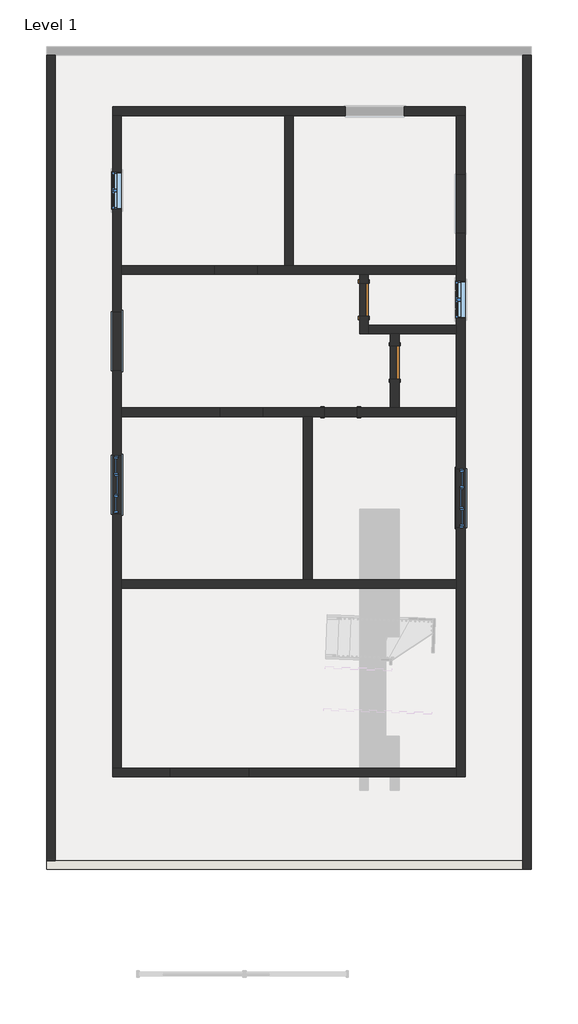
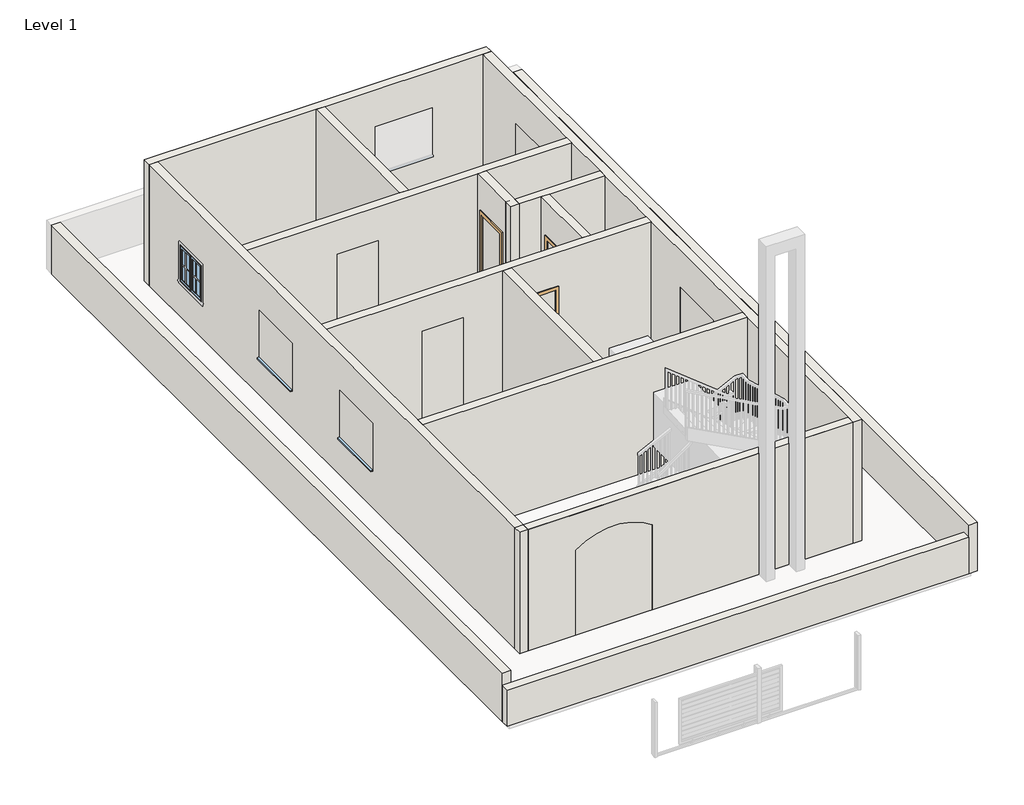
# One storey, part 1 of 4: 27 walls, 7 windows, 3 doors.
"""IFC4 building model written with IfcOpenShell, lengths in millimetres."""

from ifc_helpers import new_model, si_unit, frame, origin, origin_with_axes, place, context, project, spatial, polyline, circle_curve, outline, extrude, faceted_brep, transform, mapped, element, save
from ifc_brep_helpers import plane_surface, revolved_surface, advanced_brep
from components import door_b6acaa4e, window_c29befe5, windows_tpl_plain_1360x1210mm_e2a6c9d8

model = new_model("IFC4")

# Units and contexts
model_context = context("Model", 3, world=origin())
ifc_project = project(units=[si_unit("LENGTHUNIT", "METRE", prefix="MILLI")], contexts=[model_context])

# Site, building, storey
site = spatial("IfcSite", under=ifc_project)
building = spatial("IfcBuilding", under=site)
storey = spatial("IfcBuildingStorey", under=building, Name="Level 1", Elevation=0.0)

# Doors
placement = place(None, origin())
door_shape = door_b6acaa4e(model_context)
element("IfcDoor", 1, ObjectType="Single-Flush : 30\" x 84\"", at=placement, inside=storey, context=model_context, shape_type="MappedRepresentation", body=[
    mapped(door_shape, transform((-9158.3126504, 6947.728857, 0.0), x_axis=(0.0, -1.0, 0.0), y_axis=(1.0, 0.0, 0.0), z_axis=(0.0, 0.0, 1.0))),
])
element("IfcDoor", 2, ObjectType="Single-Flush : 30\" x 84\"", at=placement, inside=storey, context=model_context, shape_type="MappedRepresentation", body=[
    mapped(door_shape, transform((-9691.7126504, 4356.928857, 0.0), x_axis=(-1.0, 0.0, 0.0), y_axis=(0.0, -1.0, 0.0), z_axis=(0.0, 0.0, 1.0))),
])
element("IfcDoor", 3, ObjectType="Single-Flush : 30\" x 84\"", at=placement, inside=storey, context=model_context, shape_type="MappedRepresentation", body=[
    mapped(door_shape, transform((-8447.1126504, 5499.928857, 0.0), x_axis=(0.0, -1.0, 0.0), y_axis=(1.0, 0.0, 0.0), z_axis=(0.0, 0.0, 1.0))),
])

# Walls
element("IfcWall", 4, ObjectType="Generic - 4.5\" p", at=placement, inside=storey, context=model_context, shape_type="SweptSolid", body=[
    extrude(outline(polyline([(-10987.1126504, 7735.128857), (-10987.1126504, 11189.528857), (-10783.9126504, 11189.528857), (-10783.9126504, 7735.128857), (-10987.1126504, 7735.128857)])), origin_with_axes(), (0.0, 0.0, 1.0), 3048.0),
])
element("IfcWall", 5, ObjectType="Generic - 4.5\" p", at=placement, inside=storey, context=model_context, shape_type="Brep", body=[
    faceted_brep([(-7024.7126504, 7735.128857, 0.0), (-10783.9126504, 7735.128857, 0.0), (-10987.1126504, 7735.128857, 0.0), (-11604.7126504, 7735.128857, 0.0), (-11604.7126504, 7735.128857, 2200.0), (-12604.7126504, 7735.128857, 2200.0), (-12604.7126504, 7735.128857, 0.0), (-14746.3126504, 7735.128857, 0.0), (-14746.3126504, 7735.128857, 3048.0), (-10987.1126504, 7735.128857, 3048.0), (-10783.9126504, 7735.128857, 3048.0), (-7024.7126504, 7735.128857, 3048.0), (-11604.7126504, 7531.928857, 2200.0), (-11604.7126504, 7531.928857, 0.0), (-9259.9126504, 7531.928857, 0.0), (-9056.7126504, 7531.928857, 0.0), (-7024.7126504, 7531.928857, 0.0), (-7024.7126504, 7531.928857, 3048.0), (-9056.7126504, 7531.928857, 3048.0), (-9259.9126504, 7531.928857, 3048.0), (-14746.3126504, 7531.928857, 3048.0), (-14746.3126504, 7531.928857, 0.0), (-12604.7126504, 7531.928857, 0.0), (-12604.7126504, 7531.928857, 2200.0)], [[[0, 1, 2, 3, 4, 5, 6, 7, 8, 9, 10, 11]], [[12, 13, 14, 15, 16, 17, 18, 19, 20, 21, 22, 23]], [[22, 21, 7, 6]], [[16, 15, 14, 13, 3, 2, 1, 0]], [[11, 10, 9, 8, 20, 19, 18, 17]], [[8, 7, 21, 20]], [[0, 11, 17, 16]], [[4, 3, 13, 12]], [[5, 4, 12, 23]], [[6, 5, 23, 22]]]),
])
element("IfcWall", 6, ObjectType="Generic - 4.5\" p", at=placement, inside=storey, context=model_context, shape_type="Brep", body=[
    faceted_brep([(-9259.9126504, 6566.728857, 2133.6), (-9259.9126504, 6566.728857, 0.0), (-9259.9126504, 6160.328857, 0.0), (-9259.9126504, 6160.328857, 3048.0), (-9259.9126504, 7531.928857, 3048.0), (-9259.9126504, 7531.928857, 0.0), (-9259.9126504, 7328.728857, 0.0), (-9259.9126504, 7328.728857, 2133.6), (-9056.7126504, 6160.328857, 0.0), (-9056.7126504, 6363.528857, 0.0), (-9056.7126504, 6566.728857, 0.0), (-9056.7126504, 6566.728857, 2133.6), (-9056.7126504, 7328.728857, 2133.6), (-9056.7126504, 7328.728857, 0.0), (-9056.7126504, 7531.928857, 0.0), (-9056.7126504, 7531.928857, 3048.0), (-9056.7126504, 6363.528857, 3048.0), (-9056.7126504, 6160.328857, 3048.0)], [[[0, 1, 2, 3, 4, 5, 6, 7]], [[8, 9, 10, 11, 12, 13, 14, 15, 16, 17]], [[6, 5, 14, 13]], [[2, 1, 10, 9, 8]], [[4, 3, 17, 16, 15]], [[5, 4, 15, 14]], [[3, 2, 8, 17]], [[11, 10, 1, 0]], [[12, 11, 0, 7]], [[13, 12, 7, 6]]]),
])
element("IfcWall", 7, ObjectType="Generic - 4.5\" p", at=placement, inside=storey, context=model_context, shape_type="Brep", body=[
    faceted_brep([(-9056.7126504, 6160.328857, 0.0), (-8548.7126504, 6160.328857, 0.0), (-8345.5126504, 6160.328857, 0.0), (-7024.7126504, 6160.328857, 0.0), (-7024.7126504, 6160.328857, 3048.0), (-8345.5126504, 6160.328857, 3048.0), (-8548.7126504, 6160.328857, 3048.0), (-9056.7126504, 6160.328857, 3048.0), (-9056.7126504, 6363.528857, 0.0), (-9056.7126504, 6363.528857, 3048.0), (-7024.7126504, 6363.528857, 3048.0), (-7024.7126504, 6363.528857, 0.0)], [[[0, 1, 2, 3, 4, 5, 6, 7]], [[8, 9, 10, 11]], [[3, 2, 1, 0, 8, 11]], [[7, 6, 5, 4, 10, 9]], [[0, 7, 9, 8]], [[4, 3, 11, 10]]]),
])
element("IfcWall", 8, ObjectType="Generic - 4.5\" p", at=placement, inside=storey, context=model_context, shape_type="SweptSolid", body=[
    extrude(outline(polyline([(5118.928857, 2133.6), (5118.928857, 0.0), (4458.528857, 0.0), (4458.528857, 3048.0), (6160.328857, 3048.0), (6160.328857, 0.0), (5880.928857, 0.0), (5880.928857, 2133.6), (5118.928857, 2133.6)])), frame((-8548.7126504, 0.0, 0.0), z_axis=(1.0, 0.0, 0.0), x_axis=(0.0, 1.0, 0.0)), (0.0, 0.0, 1.0), 203.2),
])
element("IfcWall", 9, ObjectType="Generic - 4.5\" p", at=placement, inside=storey, context=model_context, shape_type="Brep", body=[
    faceted_brep([(-10072.7126504, 4458.528857, 2133.6), (-10072.7126504, 4458.528857, 0.0), (-11477.7126504, 4458.528857, 0.0), (-11477.7126504, 4458.528857, 2200.0), (-12477.7126504, 4458.528857, 2200.0), (-12477.7126504, 4458.528857, 0.0), (-14746.3126504, 4458.528857, 0.0), (-14746.3126504, 4458.528857, 3048.0), (-8548.7126504, 4458.528857, 3048.0), (-8345.5126504, 4458.528857, 3048.0), (-7024.7126504, 4458.528857, 3048.0), (-7024.7126504, 4458.528857, 0.0), (-8345.5126504, 4458.528857, 0.0), (-8548.7126504, 4458.528857, 0.0), (-9310.7126504, 4458.528857, 0.0), (-9310.7126504, 4458.528857, 2133.6), (-11477.7126504, 4255.328857, 0.0), (-10555.3126504, 4255.328857, 0.0), (-10352.1126504, 4255.328857, 0.0), (-10072.7126504, 4255.328857, 0.0), (-10072.7126504, 4255.328857, 2133.6), (-9310.7126504, 4255.328857, 2133.6), (-9310.7126504, 4255.328857, 0.0), (-7024.7126504, 4255.328857, 0.0), (-7024.7126504, 4255.328857, 3048.0), (-10352.1126504, 4255.328857, 3048.0), (-10555.3126504, 4255.328857, 3048.0), (-14746.3126504, 4255.328857, 3048.0), (-14746.3126504, 4255.328857, 0.0), (-12477.7126504, 4255.328857, 0.0), (-12477.7126504, 4255.328857, 2200.0), (-11477.7126504, 4255.328857, 2200.0)], [[[0, 1, 2, 3, 4, 5, 6, 7, 8, 9, 10, 11, 12, 13, 14, 15]], [[16, 17, 18, 19, 20, 21, 22, 23, 24, 25, 26, 27, 28, 29, 30, 31]], [[29, 28, 6, 5]], [[2, 1, 19, 18, 17, 16]], [[14, 13, 12, 11, 23, 22]], [[10, 9, 8, 7, 27, 26, 25, 24]], [[11, 10, 24, 23]], [[7, 6, 28, 27]], [[3, 2, 16, 31]], [[4, 3, 31, 30]], [[5, 4, 30, 29]], [[20, 19, 1, 0]], [[21, 20, 0, 15]], [[22, 21, 15, 14]]]),
])
element("IfcWall", 10, ObjectType="Generic - 4.5\" p", at=placement, inside=storey, context=model_context, shape_type="SweptSolid", body=[
    extrude(outline(polyline([(-10555.3126504, 496.128857), (-10555.3126504, 4255.328857), (-10352.1126504, 4255.328857), (-10352.1126504, 496.128857), (-10555.3126504, 496.128857)])), origin_with_axes(), (0.0, 0.0, 1.0), 3048.0),
])
element("IfcWall", 11, ObjectType="Generic - 4.5\" p", at=placement, inside=storey, context=model_context, shape_type="Brep", body=[
    faceted_brep([(-14746.3126504, 292.928857, 0.0), (-7024.7126504, 292.928857, 0.0), (-7024.7126504, 292.928857, 3048.0), (-14746.3126504, 292.928857, 3048.0), (-14746.3126504, 496.128857, 0.0), (-14746.3126504, 496.128857, 3048.0), (-10555.3126504, 496.128857, 3048.0), (-10352.1126504, 496.128857, 3048.0), (-7024.7126504, 496.128857, 3048.0), (-7024.7126504, 496.128857, 0.0), (-10352.1126504, 496.128857, 0.0), (-10555.3126504, 496.128857, 0.0)], [[[0, 1, 2, 3]], [[4, 5, 6, 7, 8, 9, 10, 11]], [[1, 0, 4, 11, 10, 9]], [[3, 2, 8, 7, 6, 5]], [[2, 1, 9, 8]], [[0, 3, 5, 4]]]),
])
element("IfcWall", 12, ObjectType="Generic - 4.5\" p", at=placement, inside=storey, context=model_context, shape_type="SweptSolid", body=[
    extrude(outline(polyline([(-10987.1126504, 7735.128857), (-10987.1126504, 11189.528857), (-10783.9126504, 11189.528857), (-10783.9126504, 7735.128857), (-10987.1126504, 7735.128857)])), origin_with_axes(), (0.0, 0.0, 1.0), 3048.0),
])
element("IfcWall", 13, ObjectType="Generic - 4.5\" p", at=placement, inside=storey, context=model_context, shape_type="Brep", body=[
    faceted_brep([(-7024.7126504, 7735.128857, 0.0), (-10783.9126504, 7735.128857, 0.0), (-10987.1126504, 7735.128857, 0.0), (-14746.3126504, 7735.128857, 0.0), (-14746.3126504, 7735.128857, 3048.0), (-10987.1126504, 7735.128857, 3048.0), (-10783.9126504, 7735.128857, 3048.0), (-7024.7126504, 7735.128857, 3048.0), (-7024.7126504, 7531.928857, 0.0), (-7024.7126504, 7531.928857, 3048.0), (-9056.7126504, 7531.928857, 3048.0), (-9259.9126504, 7531.928857, 3048.0), (-14746.3126504, 7531.928857, 3048.0), (-14746.3126504, 7531.928857, 0.0), (-9259.9126504, 7531.928857, 0.0), (-9056.7126504, 7531.928857, 0.0)], [[[0, 1, 2, 3, 4, 5, 6, 7]], [[8, 9, 10, 11, 12, 13, 14, 15]], [[3, 2, 1, 0, 8, 15, 14, 13]], [[7, 6, 5, 4, 12, 11, 10, 9]], [[4, 3, 13, 12]], [[0, 7, 9, 8]]]),
])
element("IfcWall", 14, ObjectType="Generic - 4.5\" p", at=placement, inside=storey, context=model_context, shape_type="SweptSolid", body=[
    extrude(outline(polyline([(-9259.9126504, 6363.528857), (-9259.9126504, 7531.928857), (-9056.7126504, 7531.928857), (-9056.7126504, 6363.528857), (-9259.9126504, 6363.528857)])), origin_with_axes(), (0.0, 0.0, 1.0), 3048.0),
])
element("IfcWall", 15, ObjectType="Generic - 4.5\" p", at=placement, inside=storey, context=model_context, shape_type="Brep", body=[
    faceted_brep([(-9056.7126504, 6160.328857, 0.0), (-8548.7126504, 6160.328857, 0.0), (-8345.5126504, 6160.328857, 0.0), (-7024.7126504, 6160.328857, 0.0), (-7024.7126504, 6160.328857, 3048.0), (-8345.5126504, 6160.328857, 3048.0), (-8548.7126504, 6160.328857, 3048.0), (-9056.7126504, 6160.328857, 3048.0), (-9056.7126504, 6363.528857, 0.0), (-9056.7126504, 6363.528857, 3048.0), (-7024.7126504, 6363.528857, 3048.0), (-7024.7126504, 6363.528857, 0.0)], [[[0, 1, 2, 3, 4, 5, 6, 7]], [[8, 9, 10, 11]], [[3, 2, 1, 0, 8, 11]], [[7, 6, 5, 4, 10, 9]], [[4, 3, 11, 10]], [[0, 7, 9, 8]]]),
])
element("IfcWall", 16, ObjectType="Generic - 4.5\" p", at=placement, inside=storey, context=model_context, shape_type="SweptSolid", body=[
    extrude(outline(polyline([(-8548.7126504, 4458.528857), (-8548.7126504, 6160.328857), (-8345.5126504, 6160.328857), (-8345.5126504, 4458.528857), (-8548.7126504, 4458.528857)])), origin_with_axes(), (0.0, 0.0, 1.0), 3048.0),
])
element("IfcWall", 17, ObjectType="Generic - 4.5\" p", at=placement, inside=storey, context=model_context, shape_type="Brep", body=[
    faceted_brep([(-7024.7126504, 4458.528857, 0.0), (-8345.5126504, 4458.528857, 0.0), (-8548.7126504, 4458.528857, 0.0), (-14746.3126504, 4458.528857, 0.0), (-14746.3126504, 4458.528857, 3048.0), (-8548.7126504, 4458.528857, 3048.0), (-8345.5126504, 4458.528857, 3048.0), (-7024.7126504, 4458.528857, 3048.0), (-7024.7126504, 4255.328857, 0.0), (-7024.7126504, 4255.328857, 3048.0), (-10352.1126504, 4255.328857, 3048.0), (-10555.3126504, 4255.328857, 3048.0), (-14746.3126504, 4255.328857, 3048.0), (-14746.3126504, 4255.328857, 0.0), (-10555.3126504, 4255.328857, 0.0), (-10352.1126504, 4255.328857, 0.0)], [[[0, 1, 2, 3, 4, 5, 6, 7]], [[8, 9, 10, 11, 12, 13, 14, 15]], [[3, 2, 1, 0, 8, 15, 14, 13]], [[7, 6, 5, 4, 12, 11, 10, 9]], [[0, 7, 9, 8]], [[4, 3, 13, 12]]]),
])
element("IfcWall", 18, ObjectType="Generic - 4.5\" p", at=placement, inside=storey, context=model_context, shape_type="SweptSolid", body=[
    extrude(outline(polyline([(-10555.3126504, 496.128857), (-10555.3126504, 4255.328857), (-10352.1126504, 4255.328857), (-10352.1126504, 496.128857), (-10555.3126504, 496.128857)])), origin_with_axes(), (0.0, 0.0, 1.0), 3048.0),
])
element("IfcWall", 19, ObjectType="Generic - 4.5\" p", at=placement, inside=storey, context=model_context, shape_type="Brep", body=[
    faceted_brep([(-14746.3126504, 292.928857, 0.0), (-7024.7126504, 292.928857, 0.0), (-7024.7126504, 292.928857, 3048.0), (-14746.3126504, 292.928857, 3048.0), (-14746.3126504, 496.128857, 0.0), (-14746.3126504, 496.128857, 3048.0), (-10555.3126504, 496.128857, 3048.0), (-10352.1126504, 496.128857, 3048.0), (-7024.7126504, 496.128857, 3048.0), (-7024.7126504, 496.128857, 0.0), (-10352.1126504, 496.128857, 0.0), (-10555.3126504, 496.128857, 0.0)], [[[0, 1, 2, 3]], [[4, 5, 6, 7, 8, 9, 10, 11]], [[1, 0, 4, 11, 10, 9]], [[3, 2, 8, 7, 6, 5]], [[2, 1, 9, 8]], [[0, 3, 5, 4]]]),
])
element("IfcWall", 20, ObjectType="Generic - 4.5\" p", at=placement, inside=storey, context=model_context, shape_type="Brep", body=[
    faceted_brep([(-5500.7126504, 12579.7156917, 0.0), (-5500.7126504, -5980.871143, 0.0), (-5500.7126504, -6184.071143, 0.0), (-5500.7126504, -6184.071143, 914.4), (-5500.7126504, -6184.071143, 1219.2), (-5500.7126504, 12579.7156917, 1219.2), (-5297.5126504, 12579.7156917, 0.0), (-5297.5126504, 12579.7156917, 1219.2), (-5297.5126504, -6184.071143, 1219.2), (-5297.5126504, -6184.071143, 0.0)], [[[0, 1, 2, 3, 4, 5]], [[6, 7, 8, 9]], [[2, 1, 0, 6, 9]], [[5, 4, 8, 7]], [[0, 5, 7, 6]], [[4, 3, 2, 9, 8]]]),
])
element("IfcWall", 21, ObjectType="Generic - 4.5\" p", at=placement, inside=storey, context=model_context, shape_type="Brep", body=[
    faceted_brep([(-5500.7126504, -5980.871143, 0.0), (-16270.3126504, -5980.871143, 0.0), (-16473.5126504, -5980.871143, 0.0), (-16473.5126504, -5980.871143, 914.4), (-5500.7126504, -5980.871143, 914.4), (-5500.7126504, -6184.071143, 0.0), (-5500.7126504, -6184.071143, 914.4), (-16473.5126504, -6184.071143, 914.4), (-16473.5126504, -6184.071143, 0.0)], [[[0, 1, 2, 3, 4]], [[5, 6, 7, 8]], [[2, 1, 0, 5, 8]], [[4, 3, 7, 6]], [[0, 4, 6, 5]], [[3, 2, 8, 7]]]),
])
element("IfcWall", 22, ObjectType="Generic - 4.5\" p", at=placement, inside=storey, context=model_context, shape_type="Brep", body=[
    faceted_brep([(-16270.3126504, -5980.871143, 0.0), (-16270.3126504, 12579.7156917, 0.0), (-16270.3126504, 12579.7156917, 1219.2), (-16270.3126504, -5980.871143, 1219.2), (-16473.5126504, -5980.871143, 0.0), (-16473.5126504, -5980.871143, 914.4), (-16473.5126504, -5980.871143, 1219.2), (-16473.5126504, 12579.7156917, 1219.2), (-16473.5126504, 12579.7156917, 0.0)], [[[0, 1, 2, 3]], [[4, 5, 6, 7, 8]], [[1, 0, 4, 8]], [[3, 2, 7, 6]], [[2, 1, 8, 7]], [[0, 3, 6, 5, 4]]]),
])
element("IfcWall", 23, ObjectType="Generic - 9\" w", at=placement, inside=storey, context=model_context, shape_type="Brep", body=[
    faceted_brep([(-14949.5126504, 11189.528857, 0.0), (-14746.3126504, 11189.528857, 0.0), (-10987.1126504, 11189.528857, 0.0), (-10783.9126504, 11189.528857, 0.0), (-7024.7126504, 11189.528857, 0.0), (-6821.5126504, 11189.528857, 0.0), (-6821.5126504, 11189.528857, 3048.0), (-7024.7126504, 11189.528857, 3048.0), (-10783.9126504, 11189.528857, 3048.0), (-10987.1126504, 11189.528857, 3048.0), (-14746.3126504, 11189.528857, 3048.0), (-14949.5126504, 11189.528857, 3048.0), (-8224.3126504, 11189.528857, 2124.4), (-8224.3126504, 11189.528857, 914.4), (-9584.3126504, 11189.528857, 914.4), (-9584.3126504, 11189.528857, 2124.4), (-14949.5126504, 11392.728857, 0.0), (-14949.5126504, 11392.728857, 3048.0), (-6821.5126504, 11392.728857, 3048.0), (-6821.5126504, 11392.728857, 0.0), (-8224.3126504, 11392.728857, 2124.4), (-9584.3126504, 11392.728857, 2124.4), (-9584.3126504, 11392.728857, 914.4), (-8224.3126504, 11392.728857, 914.4)], [[[0, 1, 2, 3, 4, 5, 6, 7, 8, 9, 10, 11], [12, 13, 14, 15]], [[16, 17, 18, 19], [20, 21, 22, 23]], [[5, 4, 3, 2, 1, 0, 16, 19]], [[11, 10, 9, 8, 7, 6, 18, 17]], [[6, 5, 19, 18]], [[0, 11, 17, 16]], [[13, 12, 20, 23]], [[14, 13, 23, 22]], [[15, 14, 22, 21]], [[12, 15, 21, 20]]]),
])
element("IfcWall", 24, ObjectType="Generic - 9\" w", at=placement, inside=storey, context=model_context, shape_type="Brep", body=[
    faceted_brep([(-7024.7126504, 11189.528857, 0.0), (-7024.7126504, 7735.128857, 0.0), (-7024.7126504, 7531.928857, 0.0), (-7024.7126504, 6363.528857, 0.0), (-7024.7126504, 6160.328857, 0.0), (-7024.7126504, 4458.528857, 0.0), (-7024.7126504, 4255.328857, 0.0), (-7024.7126504, 496.128857, 0.0), (-7024.7126504, 292.928857, 0.0), (-7024.7126504, -3847.271143, 0.0), (-7024.7126504, -4050.471143, 0.0), (-7024.7126504, -4050.471143, 3048.0), (-7024.7126504, -3847.271143, 3048.0), (-7024.7126504, 292.928857, 3048.0), (-7024.7126504, 496.128857, 3048.0), (-7024.7126504, 4255.328857, 3048.0), (-7024.7126504, 4458.528857, 3048.0), (-7024.7126504, 6160.328857, 3048.0), (-7024.7126504, 6363.528857, 3048.0), (-7024.7126504, 7531.928857, 3048.0), (-7024.7126504, 7735.128857, 3048.0), (-7024.7126504, 11189.528857, 3048.0), (-7024.7126504, 8477.528857, 2124.4), (-7024.7126504, 8477.528857, 914.4), (-7024.7126504, 9837.528857, 914.4), (-7024.7126504, 9837.528857, 2124.4), (-7024.7126504, 3055.728857, 2124.4), (-7024.7126504, 1695.728857, 2124.4), (-7024.7126504, 1695.728857, 914.4), (-7024.7126504, 3055.728857, 914.4), (-7024.7126504, 7379.528857, 1828.8), (-7024.7126504, 6515.928857, 1828.8), (-7024.7126504, 6515.928857, 914.4), (-7024.7126504, 7379.528857, 914.4), (-6821.5126504, 11189.528857, 0.0), (-6821.5126504, 11189.528857, 3048.0), (-6821.5126504, -4050.471143, 3048.0), (-6821.5126504, -4050.471143, 0.0), (-6821.5126504, 8477.528857, 2124.4), (-6821.5126504, 9837.528857, 2124.4), (-6821.5126504, 9837.528857, 914.4), (-6821.5126504, 8477.528857, 914.4), (-6821.5126504, 3055.728857, 2124.4), (-6821.5126504, 3055.728857, 914.4), (-6821.5126504, 1695.728857, 914.4), (-6821.5126504, 1695.728857, 2124.4), (-6821.5126504, 7379.528857, 1828.8), (-6821.5126504, 7379.528857, 914.4), (-6821.5126504, 6515.928857, 914.4), (-6821.5126504, 6515.928857, 1828.8)], [[[0, 1, 2, 3, 4, 5, 6, 7, 8, 9, 10, 11, 12, 13, 14, 15, 16, 17, 18, 19, 20, 21], [22, 23, 24, 25], [26, 27, 28, 29], [30, 31, 32, 33]], [[34, 35, 36, 37], [38, 39, 40, 41], [42, 43, 44, 45], [46, 47, 48, 49]], [[10, 9, 8, 7, 6, 5, 4, 3, 2, 1, 0, 34, 37]], [[21, 20, 19, 18, 17, 16, 15, 14, 13, 12, 11, 36, 35]], [[0, 21, 35, 34]], [[11, 10, 37, 36]], [[23, 22, 38, 41]], [[24, 23, 41, 40]], [[25, 24, 40, 39]], [[22, 25, 39, 38]], [[43, 42, 26, 29]], [[44, 43, 29, 28]], [[45, 44, 28, 27]], [[42, 45, 27, 26]], [[47, 46, 30, 33]], [[48, 47, 33, 32]], [[49, 48, 32, 31]], [[46, 49, 31, 30]]]),
])
element("IfcWall", 25, ObjectType="Generic - 9\" w", at=placement, inside=storey, context=model_context, shape_type="AdvancedBrep", body=[
    advanced_brep(
    [(-14949.5126504, -3847.271143, 3048.0), (-14746.3126504, -3847.271143, 3048.0), (-7024.7126504, -3847.271143, 3048.0), (-7024.7126504, -3847.271143, 0.0), (-11799.9126504, -3847.271143, 0.0), (-11799.9126504, -3847.271143, 2133.6), (-13628.7126504, -3847.271143, 2133.6), (-13628.7126504, -3847.271143, 0.0), (-14746.3126504, -3847.271143, 0.0), (-14949.5126504, -3847.271143, 0.0), (-7024.7126504, -4050.471143, 3048.0), (-14949.5126504, -4050.471143, 3048.0), (-14949.5126504, -4050.471143, 0.0), (-13628.7126504, -4050.471143, 0.0), (-13628.7126504, -4050.471143, 2133.6), (-11799.9126504, -4050.471143, 2133.6), (-11799.9126504, -4050.471143, 0.0), (-7024.7126504, -4050.471143, 0.0)],
    [
        (0, 1),
        (1, 2),
        (2, 3),
        (3, 4),
        (4, 5),
        (5, 6, circle_curve(frame((-12714.3126504, -3847.271143, 917.0443508), z_axis=(0.0, -1.0, 0.0), x_axis=(1.0, 0.0, 0.0)), 1521.8853464)),
        (6, 7),
        (7, 8),
        (8, 9),
        (9, 0),
        (10, 11),
        (11, 12),
        (12, 13),
        (13, 14),
        (14, 15, circle_curve(frame((-12714.3126504, -4050.471143, 917.0443508), z_axis=(0.0, 1.0, 0.0), x_axis=(1.0, 0.0, 0.0)), 1521.8853464)),
        (15, 16),
        (16, 17),
        (17, 10),
        (3, 17),
        (16, 4),
        (12, 9),
        (7, 13),
        (0, 11),
        (10, 2),
        (15, 5),
        (14, 6),
    ],
    [
        plane_surface(frame((-6923.1126504, -3847.271143, 0.0), z_axis=(0.0, 1.0, 0.0), x_axis=(-1.0, 0.0, 0.0))),
        plane_surface(frame((-6923.1126504, -4050.471143, 0.0), z_axis=(0.0, -1.0, 0.0), x_axis=(1.0, 0.0, 0.0))),
        plane_surface(frame((-6923.1126504, -3847.271143, 0.0), z_axis=(0.0, 0.0, -1.0), x_axis=(0.0, -1.0, 0.0))),
        plane_surface(frame((-14847.9126504, -3847.271143, 3048.0), z_axis=(0.0, 0.0, 1.0), x_axis=(0.0, -1.0, 0.0))),
        plane_surface(frame((-7024.7126504, 11291.128857, 0.0), z_axis=(1.0, 0.0, 0.0), x_axis=(0.0, -1.0, 0.0))),
        plane_surface(frame((-14949.5126504, -3948.871143, 0.0), z_axis=(-1.0, 0.0, 0.0), x_axis=(0.0, -1.0, 0.0))),
        plane_surface(frame((-11799.9126504, -5574.471143, 0.0), z_axis=(-1.0, 0.0, 0.0), x_axis=(0.0, 1.0, 0.0))),
        revolved_surface(polyline([(-11192.427303999999, -4050.471143, 917.0443508), (-11192.427303999999, -3847.271143, 917.0443508)]), (-12714.3126504, -2526.471143, 917.0443508), (0.0, -1.0, 0.0)),
        plane_surface(frame((-13628.7126504, -5574.471143, 2133.6), z_axis=(1.0, 0.0, 0.0), x_axis=(0.0, 1.0, 0.0))),
    ],
    [
        (0, [[1, 2, 3, 4, 5, 6, 7, 8, 9, 10]]),
        (1, [[11, 12, 13, 14, 15, 16, 17, 18]]),
        (2, [[19, -17, 20, -4]]),
        (2, [[21, -9, -8, 22, -13]]),
        (3, [[-2, -1, 23, -11, 24]]),
        (4, [[-3, -24, -18, -19]]),
        (5, [[-10, -21, -12, -23]]),
        (6, [[25, -5, -20, -16]]),
        (7, [[-25, -15, 26, -6]]),
        (8, [[-26, -14, -22, -7]]),
    ],
),
])
element("IfcWall", 26, ObjectType="Generic - 9\" w", at=placement, inside=storey, context=model_context, shape_type="Brep", body=[
    faceted_brep([(-14746.3126504, -3847.271143, 0.0), (-14746.3126504, 292.928857, 0.0), (-14746.3126504, 496.128857, 0.0), (-14746.3126504, 4255.328857, 0.0), (-14746.3126504, 4458.528857, 0.0), (-14746.3126504, 7531.928857, 0.0), (-14746.3126504, 7735.128857, 0.0), (-14746.3126504, 11189.528857, 0.0), (-14746.3126504, 11189.528857, 3048.0), (-14746.3126504, 7735.128857, 3048.0), (-14746.3126504, 7531.928857, 3048.0), (-14746.3126504, 4458.528857, 3048.0), (-14746.3126504, 4255.328857, 3048.0), (-14746.3126504, 496.128857, 3048.0), (-14746.3126504, 292.928857, 3048.0), (-14746.3126504, -3847.271143, 3048.0), (-14746.3126504, 5315.228857, 2124.4), (-14746.3126504, 6675.228857, 2124.4), (-14746.3126504, 6675.228857, 914.4), (-14746.3126504, 5315.228857, 914.4), (-14746.3126504, 2000.528857, 2124.4), (-14746.3126504, 3360.528857, 2124.4), (-14746.3126504, 3360.528857, 914.4), (-14746.3126504, 2000.528857, 914.4), (-14746.3126504, 9894.128857, 1828.8), (-14746.3126504, 9894.128857, 914.4), (-14746.3126504, 9030.528857, 914.4), (-14746.3126504, 9030.528857, 1828.8), (-14949.5126504, -3847.271143, 0.0), (-14949.5126504, -3847.271143, 3048.0), (-14949.5126504, 11189.528857, 3048.0), (-14949.5126504, 11189.528857, 0.0), (-14949.5126504, 5315.228857, 2124.4), (-14949.5126504, 5315.228857, 914.4), (-14949.5126504, 6675.228857, 914.4), (-14949.5126504, 6675.228857, 2124.4), (-14949.5126504, 2000.528857, 2124.4), (-14949.5126504, 2000.528857, 914.4), (-14949.5126504, 3360.528857, 914.4), (-14949.5126504, 3360.528857, 2124.4), (-14949.5126504, 9894.128857, 1828.8), (-14949.5126504, 9030.528857, 1828.8), (-14949.5126504, 9030.528857, 914.4), (-14949.5126504, 9894.128857, 914.4)], [[[0, 1, 2, 3, 4, 5, 6, 7, 8, 9, 10, 11, 12, 13, 14, 15], [16, 17, 18, 19], [20, 21, 22, 23], [24, 25, 26, 27]], [[28, 29, 30, 31], [32, 33, 34, 35], [36, 37, 38, 39], [40, 41, 42, 43]], [[7, 6, 5, 4, 3, 2, 1, 0, 28, 31]], [[15, 14, 13, 12, 11, 10, 9, 8, 30, 29]], [[8, 7, 31, 30]], [[0, 15, 29, 28]], [[33, 32, 16, 19]], [[34, 33, 19, 18]], [[35, 34, 18, 17]], [[32, 35, 17, 16]], [[37, 36, 20, 23]], [[38, 37, 23, 22]], [[39, 38, 22, 21]], [[36, 39, 21, 20]], [[25, 24, 40, 43]], [[26, 25, 43, 42]], [[27, 26, 42, 41]], [[24, 27, 41, 40]]]),
])
element("IfcWall", 27, ObjectType="Generic - 9\" w", at=placement, inside=storey, context=model_context, shape_type="Brep", body=[
    faceted_brep([(-7024.7126504, 11189.528857, 0.0), (-7024.7126504, 7735.128857, 0.0), (-7024.7126504, 7531.928857, 0.0), (-7024.7126504, 6363.528857, 0.0), (-7024.7126504, 6160.328857, 0.0), (-7024.7126504, 4458.528857, 0.0), (-7024.7126504, 4255.328857, 0.0), (-7024.7126504, 496.128857, 0.0), (-7024.7126504, 292.928857, 0.0), (-7024.7126504, -3847.271143, 0.0), (-7024.7126504, -3847.271143, 3048.0), (-7024.7126504, 292.928857, 3048.0), (-7024.7126504, 496.128857, 3048.0), (-7024.7126504, 4255.328857, 3048.0), (-7024.7126504, 4458.528857, 3048.0), (-7024.7126504, 6160.328857, 3048.0), (-7024.7126504, 6363.528857, 3048.0), (-7024.7126504, 7531.928857, 3048.0), (-7024.7126504, 7735.128857, 3048.0), (-7024.7126504, 11189.528857, 3048.0), (-7024.7126504, 7379.528857, 1828.8), (-7024.7126504, 6515.928857, 1828.8), (-7024.7126504, 6515.928857, 914.4), (-7024.7126504, 7379.528857, 914.4), (-6821.5126504, 11189.528857, 0.0), (-6821.5126504, 11189.528857, 3048.0), (-6821.5126504, -3847.271143, 3048.0), (-6821.5126504, -3847.271143, 0.0), (-6821.5126504, 7379.528857, 1828.8), (-6821.5126504, 7379.528857, 914.4), (-6821.5126504, 6515.928857, 914.4), (-6821.5126504, 6515.928857, 1828.8)], [[[0, 1, 2, 3, 4, 5, 6, 7, 8, 9, 10, 11, 12, 13, 14, 15, 16, 17, 18, 19], [20, 21, 22, 23]], [[24, 25, 26, 27], [28, 29, 30, 31]], [[9, 8, 7, 6, 5, 4, 3, 2, 1, 0, 24, 27]], [[19, 18, 17, 16, 15, 14, 13, 12, 11, 10, 26, 25]], [[29, 28, 20, 23]], [[30, 29, 23, 22]], [[31, 30, 22, 21]], [[28, 31, 21, 20]], [[0, 19, 25, 24]], [[10, 9, 27, 26]]]),
])
element("IfcWall", 28, ObjectType="Generic - 9\" w", at=placement, inside=storey, context=model_context, shape_type="SweptSolid", body=[
    extrude(outline(polyline([(-14746.3126504, -3847.271143), (-7024.7126504, -3847.271143), (-7024.7126504, -4050.471143), (-14746.3126504, -4050.471143), (-14746.3126504, -3847.271143)])), origin_with_axes(), (0.0, 0.0, 1.0), 3048.0),
])
element("IfcWall", 29, ObjectType="Generic - 9\" w", at=placement, inside=storey, context=model_context, shape_type="Brep", body=[
    faceted_brep([(-14746.3126504, -3847.271143, 0.0), (-14746.3126504, 292.928857, 0.0), (-14746.3126504, 496.128857, 0.0), (-14746.3126504, 4255.328857, 0.0), (-14746.3126504, 4458.528857, 0.0), (-14746.3126504, 7531.928857, 0.0), (-14746.3126504, 7735.128857, 0.0), (-14746.3126504, 11189.528857, 0.0), (-14746.3126504, 11189.528857, 3048.0), (-14746.3126504, 7735.128857, 3048.0), (-14746.3126504, 7531.928857, 3048.0), (-14746.3126504, 4458.528857, 3048.0), (-14746.3126504, 4255.328857, 3048.0), (-14746.3126504, 496.128857, 3048.0), (-14746.3126504, 292.928857, 3048.0), (-14746.3126504, -3847.271143, 3048.0), (-14746.3126504, 9894.128857, 1828.8), (-14746.3126504, 9894.128857, 914.4), (-14746.3126504, 9030.528857, 914.4), (-14746.3126504, 9030.528857, 1828.8), (-14949.5126504, -3847.271143, 0.0), (-14949.5126504, -3847.271143, 3048.0), (-14949.5126504, 11189.528857, 3048.0), (-14949.5126504, 11189.528857, 0.0), (-14949.5126504, 9894.128857, 1828.8), (-14949.5126504, 9030.528857, 1828.8), (-14949.5126504, 9030.528857, 914.4), (-14949.5126504, 9894.128857, 914.4)], [[[0, 1, 2, 3, 4, 5, 6, 7, 8, 9, 10, 11, 12, 13, 14, 15], [16, 17, 18, 19]], [[20, 21, 22, 23], [24, 25, 26, 27]], [[7, 6, 5, 4, 3, 2, 1, 0, 20, 23]], [[15, 14, 13, 12, 11, 10, 9, 8, 22, 21]], [[17, 16, 24, 27]], [[18, 17, 27, 26]], [[19, 18, 26, 25]], [[16, 19, 25, 24]], [[8, 7, 23, 22]], [[0, 15, 21, 20]]]),
])
element("IfcWall", 30, ObjectType="Generic - 9\" w", at=placement, inside=storey, context=model_context, shape_type="SweptSolid", body=[
    extrude(outline(polyline([(-14746.3126504, -3847.271143), (-7024.7126504, -3847.271143), (-7024.7126504, -4050.471143), (-14746.3126504, -4050.471143), (-14746.3126504, -3847.271143)])), origin_with_axes(), (0.0, 0.0, 1.0), 3048.0),
])

# Windows
window_shape = window_c29befe5(model_context)
element("IfcWindow", 31, ObjectType="Window-Casement-Double : 34\" x 36\"", at=placement, inside=storey, context=model_context, shape_type="MappedRepresentation", body=[
    mapped(window_shape, transform((-14847.9126504, 9462.328857, 0.0), x_axis=(0.0, 1.0, 0.0), y_axis=(-1.0, 0.0, 0.0), z_axis=(0.0, 0.0, 1.0))),
])
element("IfcWindow", 32, ObjectType="Window-Casement-Double : 34\" x 36\"", at=placement, inside=storey, context=model_context, shape_type="MappedRepresentation", body=[
    mapped(window_shape, transform((-6923.1126504, 6947.728857, 0.0), x_axis=(0.0, 1.0, 0.0), y_axis=(-1.0, 0.0, 0.0), z_axis=(0.0, 0.0, 1.0))),
])
element("IfcWindow", 33, ObjectType="Window-Casement-Double : 34\" x 36\"", at=placement, inside=storey, context=model_context, shape_type="MappedRepresentation", body=[
    mapped(window_shape, transform((-14847.9126504, 9462.328857, 0.0), x_axis=(0.0, 1.0, 0.0), y_axis=(-1.0, 0.0, 0.0), z_axis=(0.0, 0.0, 1.0))),
])
element("IfcWindow", 34, ObjectType="Window-Casement-Double : 34\" x 36\"", at=placement, inside=storey, context=model_context, shape_type="MappedRepresentation", body=[
    mapped(window_shape, transform((-6923.1126504, 6947.728857, 0.0), x_axis=(0.0, 1.0, 0.0), y_axis=(-1.0, 0.0, 0.0), z_axis=(0.0, 0.0, 1.0))),
])
windows_tpl_plain_1360x1210mm_shape = windows_tpl_plain_1360x1210mm_e2a6c9d8(model_context)
element("IfcWindow", 35, ObjectType="Windows_Tpl_Plain : 1360x1210mm", at=placement, inside=storey, context=model_context, shape_type="MappedRepresentation", body=[
    mapped(windows_tpl_plain_1360x1210mm_shape, transform((-6931.5692182, 1874.0621903, 14.4), x_axis=(0.0, -1.0, 0.0), y_axis=(1.0, 0.0, 0.0), z_axis=(0.0, 0.0, 1.0))),
])
element("IfcWindow", 36, ObjectType="Windows_Tpl_Plain : 1360x1210mm", at=placement, inside=storey, context=model_context, shape_type="MappedRepresentation", body=[
    mapped(windows_tpl_plain_1360x1210mm_shape, transform((-14839.4560825, 6496.8955236, 14.4), x_axis=(0.0, 1.0, 0.0), y_axis=(-1.0, 0.0, 0.0), z_axis=(0.0, 0.0, 1.0))),
])
element("IfcWindow", 37, ObjectType="Windows_Tpl_Plain : 1360x1210mm", at=placement, inside=storey, context=model_context, shape_type="MappedRepresentation", body=[
    mapped(windows_tpl_plain_1360x1210mm_shape, transform((-14839.4560825, 3182.1955236, 14.4), x_axis=(0.0, 1.0, 0.0), y_axis=(-1.0, 0.0, 0.0), z_axis=(0.0, 0.0, 1.0))),
])

save(model, "model.ifc")

# Revit data of these elements
# Type "Single-Flush : 30\" x 84\""
#   Type Mark = "4"
#   Construction Type Id = "MDOOR"
#   Assembly Code = "C1020"
#   Analytic Construction = "Metal"
#   Thickness = 0' - 2"
#   Heat Transfer Coefficient (U) = 0.651978 BTU/(h·ft²·°F)
#   Height = 7' - 0"
#   Trim Projection Ext = 0' - 1"
#   Trim Projection Int = 0' - 1"
#   Trim Width = 0' - 3"
#   Width = 2' - 6"
#   Define Thermal Properties by = 1
#   Define Thermal Properties by = 1
#   Door Material = Door - Panel
#   Frame Material = Door - Frame
#   Visual Light Transmittance = 0
#   Solar Heat Gain Coefficient = 0
#   Function = (empty or 0)
#   Wall Closure = (empty or 0)
# Type "Generic - 4.5\" p"
#   Assembly Code = "B2010"
#   Layers, outside or top first: 0' - 8" "Brick, Common" (function 1)
# Type "Generic - 9\" w"
#   Assembly Code = "B2010"
#   Layers, outside or top first: 0' - 8" no material (function 1)
# Type "Window-Casement-Double : 34\" x 36\""
#   Type Mark = "14"
#   Fire Rating = "0.5h"
#   Assembly Code = "B2020100"
#   Analytic Construction = "Double glazing - domestic"
#   Frame Extension [instance default] = 0' - 0 1/4"
#   Window Inset [instance default] = 0' - 0"
#   Wall Thickness [instance default] = 0' - 6"
#   Interior Wall Closure [instance default] = 0' - 2 1/4"
#   Half Width = 1' - 5"
#   Visual Light Transmittance = 0.81
#   Thermal Resistance (R) = 1.8146 (h·ft²·°F)/BTU
#   Solar Heat Gain Coefficient = 0.76
#   Rough Width = 2' - 10 1/2"
#   Rough Height = 3' - 0 1/2"
#   Height = 3' - 0"
#   Heat Transfer Coefficient (U) = 0.5511 BTU/(h·ft²·°F)
#   Exterior Wall Closure [instance default] = 0' - 1 1/4"
#   Extension Jamb [instance default] = 0' - 2 1/4"
#   Default Sill Height = 3' - 0"
#   Width = 2' - 10"
#   Define Thermal Properties by = 0
#   Muntin Visibility = yes
#   Interior Trim Visibility [instance default] = yes
#   Exterior Trim Visibility [instance default] = yes
#   Extension Jamb Visibility [instance default] = yes
#   Interior Trim Material = Wood - Stained
#   Muntin Pattern = Muntin Pattern_2x2 : Muntin Pattern_2x2
#   Interior Trim = Trim-Window-Interior-Flat : Picture Frame
#   Interior Frame Material = Wood - Stained
#   Glass Panel Material = Glass
#   Exterior Trim Material = Clad - White
#   Exterior Trim = Trim-Window-Exterior-Flat : with Sill
#   Exterior Frame Material = Clad - White
#   Wall Closure = (empty or 0)
# Type "Windows_Tpl_Plain : 1360x1210mm"
#   Type Mark = "21"
#   Operation = "TriplePanelVertical"
#   Construction Type Id = "GSP4R"
#   Manufacturer = "Revit"
#   Keynote = "L10"
#   Analytic Construction = "1/8 in Pilkington single glazing"
#   Wrap Layers (Ext) from Ext = 0' - 4.03543"
#   Wrap Layers (Int) from Ext = 0' - 6.98819"
#   Window Board Projection = 0' - 0.98425"
#   Window Board Extension = 0' - 0.98425"
#   Visual Light Transmittance = 0.9
#   Solar Heat Gain Coefficient = 0.78
#   Rough Width = 4' - 5.54331"
#   Rough Height = 3' - 11.6378"
#   Height = 3' - 11.6378"
#   Width = 4' - 5.54331"
#   Heat Transfer Coefficient (U) = 0.6496 BTU/(h·ft²·°F)
#   Glazing Thickness = 0' - 0.94488"
#   FrameOffset - External = 0' - 1.9685"
#   Frame Depth = 0' - 2.55906"
#   Default Head Height = 6' - 11.07087"
#   Cill Depth = 0' - 3.44488"
#   Cavity Closer Width = 0' - 1.9685"
#   Cavity Closer Offset from Ext = 0' - 4.03543"
#   Cavity Closer Depth = 0' - 3.34646"
#   Vis - Cavity Closers = yes
#   Define Thermal Properties by = 1
#   Material Trim = Window Frame
#   Material Glass = Glass
#   Material Frame = Window Frame
#   Wall Closure = (empty or 0)
# Elements 1, 2, 3 (IfcDoor, "Single-Flush : 30\" x 84\"")
#   Phase Created = New Construction
#   Materials on its faces: "Door - Frame", "Door - Panel"
# Elements 4, 5, 6, 8, 9, 10, 11, 12, 13, 14, 16, 17, 18, 19 (IfcWall, "Generic - 4.5\" p")
#   Top Offset = 0' - 0"
#   Base Offset = 0' - 0"
#   wall height = 10' - 0"
#   Phase Created = New Construction
#   Base Constraint = Level 1
#   Top Constraint = Level 2
#   Materials on its faces: "Brick, Common", "Cherry"
# Elements 7, 15 (IfcWall, "Generic - 4.5\" p")
#   Top Offset = 0' - 0"
#   Base Offset = 0' - 0"
#   wall height = 10' - 0"
#   Phase Created = New Construction
#   Base Constraint = Level 1
#   Top Constraint = Level 2
#   Materials on its faces: "Brick, Common"
# Element 20 (IfcWall, "Generic - 4.5\" p")
#   Top Offset = 0' - 0"
#   Base Offset = 0' - 0"
#   Unconnected Height = 4' - 0"
#   wall height = 4' - 0"
#   Phase Created = New Construction
#   Base Constraint = Level 1
#   Materials on its faces: "Brick, Common", "Aluminum", "Analytical Wall Surface"
# Element 21 (IfcWall, "Generic - 4.5\" p")
#   Top Offset = 0' - 0"
#   Base Offset = 0' - 0"
#   Unconnected Height = 3' - 0"
#   wall height = 3' - 0"
#   Phase Created = New Construction
#   Base Constraint = Level 1
#   Materials on its faces: "Brick, Common", "Analytical Wall Surface", "Aluminum"
# Element 22 (IfcWall, "Generic - 4.5\" p")
#   Top Offset = 0' - 0"
#   Base Offset = 0' - 0"
#   Unconnected Height = 4' - 0"
#   wall height = 4' - 0"
#   Phase Created = New Construction
#   Base Constraint = Level 1
#   Materials on its faces: "Brick, Common", "Aluminum"
# Elements 23, 24, 26, 27 (IfcWall, "Generic - 9\" w")
#   Top Offset = 0' - 0"
#   Base Offset = 0' - 0"
#   wall height = 10' - 0"
#   Phase Created = New Construction
#   Base Constraint = Level 1
#   Top Constraint = Level 2
#   Materials on its faces: "Default Wall", "Cherry"
# Element 25 (IfcWall, "Generic - 9\" w")
#   Top Offset = 0' - 0"
#   Base Offset = 0' - 0"
#   wall height = 10' - 0"
#   Phase Created = New Construction
#   Base Constraint = Level 1
#   Top Constraint = Level 2
#   Materials on its faces: "Default Wall"
# Element 28 (IfcWall, "Generic - 9\" w")
#   Top Offset = 0' - 0"
#   Base Offset = 0' - 0"
#   wall height = 10' - 0"
#   Phase Created = New Construction
#   Base Constraint = Level 1
#   Top Constraint = Level 2
#   Materials on its faces: "Default Wall", "Analytical Wall Surface"
# Element 29 (IfcWall, "Generic - 9\" w")
#   Top Offset = 0' - 0"
#   Base Offset = 0' - 0"
#   wall height = 10' - 0"
#   Phase Created = New Construction
#   Base Constraint = Level 1
#   Top Constraint = Level 2
#   Materials on its faces: "Default Wall", "Cherry", "Default Mass Exterior Wall"
# Element 30 (IfcWall, "Generic - 9\" w")
#   Top Offset = 0' - 0"
#   Base Offset = 0' - 0"
#   wall height = 10' - 0"
#   Phase Created = New Construction
#   Base Constraint = Level 1
#   Top Constraint = Level 2
#   Materials on its faces: "Default Wall", "Brick, Common"
# Element 31 (IfcWindow, "Window-Casement-Double : 34\" x 36\"")
#   Mark = "6"
#   Window Inset = 0' - 0"
#   Interior Wall Closure = 0' - 2 1/4"
#   Frame Extension = 0' - 0 1/4"
#   Exterior Wall Closure = 0' - 1 1/4"
#   Interior Trim Visibility = yes
#   Exterior Trim Visibility = yes
#   Phase Created = New Construction
#   Materials on its faces: "Wood - Stained", "Glass", "Clad - White"
# Element 32 (IfcWindow, "Window-Casement-Double : 34\" x 36\"")
#   Mark = "7"
#   Window Inset = 0' - 0"
#   Interior Wall Closure = 0' - 2 1/4"
#   Frame Extension = 0' - 0 1/4"
#   Exterior Wall Closure = 0' - 1 1/4"
#   Interior Trim Visibility = yes
#   Exterior Trim Visibility = yes
#   Phase Created = New Construction
#   Materials on its faces: "Wood - Stained", "Glass", "Clad - White"
# Element 33 (IfcWindow, "Window-Casement-Double : 34\" x 36\"")
#   Mark = "20"
#   Window Inset = 0' - 0"
#   Interior Wall Closure = 0' - 2 1/4"
#   Frame Extension = 0' - 0 1/4"
#   Exterior Wall Closure = 0' - 1 1/4"
#   Interior Trim Visibility = yes
#   Exterior Trim Visibility = yes
#   Phase Created = New Construction
#   Materials on its faces: "Wood - Stained", "Glass", "Clad - White"
# Element 34 (IfcWindow, "Window-Casement-Double : 34\" x 36\"")
#   Mark = "21"
#   Window Inset = 0' - 0"
#   Interior Wall Closure = 0' - 2 1/4"
#   Frame Extension = 0' - 0 1/4"
#   Exterior Wall Closure = 0' - 1 1/4"
#   Interior Trim Visibility = yes
#   Exterior Trim Visibility = yes
#   Phase Created = New Construction
#   Materials on its faces: "Wood - Stained", "Glass", "Clad - White"
# Element 35 (IfcWindow, "Windows_Tpl_Plain : 1360x1210mm")
#   Mark = "3"
#   Phase Created = New Construction
#   Materials on its faces: "Window Frame", "Glass"
# Element 36 (IfcWindow, "Windows_Tpl_Plain : 1360x1210mm")
#   Mark = "4"
#   Phase Created = New Construction
#   Materials on its faces: "Window Frame", "Glass"
# Element 37 (IfcWindow, "Windows_Tpl_Plain : 1360x1210mm")
#   Mark = "5"
#   Phase Created = New Construction
#   Materials on its faces: "Window Frame", "Glass"
# Materials
#   "Door - Panel": class "Wood", colour RGB 210 159 95, transparency 0, Cost = 0
#   "Door - Frame": colour RGB 118 70 51, transparency 0, Cost = 0
#   "Brick, Common": class "Masonry", colour RGB 128 0 128, transparency 0, Description = "Common brick", Cost = 0
#   "Wood - Stained": class "Wood", colour RGB 224 178 126, transparency 0, Cost = 0
#   "Glass": class "Glass", colour RGB 0 128 192, transparency 0.75, Description = "Soda Lime Glass", Cost = 0
#   "Clad - White": class "Wood", colour RGB 242 242 238, transparency 0, Cost = 0
#   "Window Frame": colour RGB 249 249 249, transparency 0
#   "Cherry": class "Wood", colour RGB 226 177 128, transparency 0, Description = "Prunus Serotina", Cost = 0
#   "Aluminum": class "Metal", colour RGB 247 247 247, transparency 0, Description = "Aluminum 6061", Cost = 0
#   "Analytical Wall Surface": class "Generic", colour RGB 0 200 200, transparency 0.5, Cost = 0
#   "Default Wall": colour RGB 128 128 128, transparency 0, Cost = 0
#   "Default Mass Exterior Wall": class "Generic", colour RGB 133 178 44, transparency 0.2, Cost = 0
